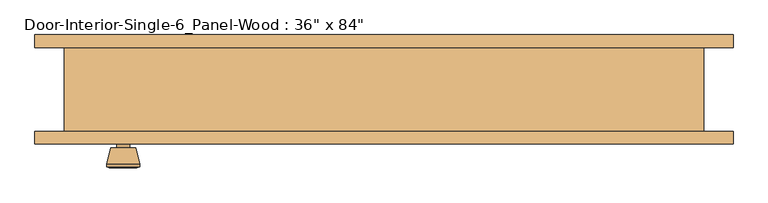
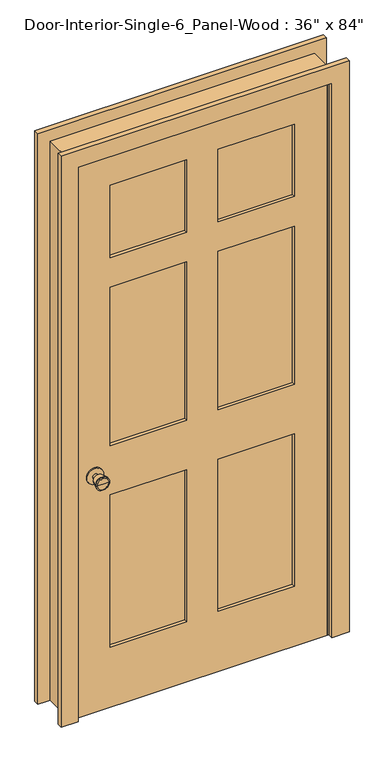
"""IFC4 building model written with IfcOpenShell, lengths in millimetres: door geometry."""

from ifc_helpers import new_model, si_unit, point, frame, frame_2d, origin, place, context, project, spatial, polyline, circle_curve, trimmed, segment, composite_curve, outline, extrude, faceted_brep, source, transform, mapped, element, save
from ifc_brep_helpers import plane_surface, cylinder_surface, revolved_surface, advanced_brep


def door_c610b25b(model_context):
    return source(origin(), model_context, "Body", "SolidModel", [
        advanced_brep(
        [(-393.7, -19.4, 914.4), (-403.7, -19.4, 914.4), (-383.7, -19.4, 914.4), (-373.2241324, 29.6, 914.4), (-414.1758676, 29.6, 914.4), (-393.7, 29.6, 914.4), (-368.7, 27.7721319, 914.4), (-418.7, 27.7721319, 914.4), (-368.7, 24.3084537, 914.4), (-418.7, 24.3084537, 914.4), (-375.063764, -0.4, 914.4), (-412.336236, -0.4, 914.4), (-383.7, -0.4, 914.4), (-403.7, -0.4, 914.4)],
        [
            (0, 1),
            (1, 2, circle_curve(frame((-393.7, -19.4, 914.4), z_axis=(0.0, -1.0, 0.0), x_axis=(-1.0, 0.0, 0.0)), 10.0)),
            (2, 0),
            (2, 1, circle_curve(frame((-393.7, -19.4, 914.4), z_axis=(0.0, -1.0, 0.0), x_axis=(-1.0, 0.0, 0.0)), 10.0)),
            (3, 4, circle_curve(frame((-393.7, 29.6, 914.4), z_axis=(0.0, 1.0, 0.0), x_axis=(-1.0, 0.0, 0.0)), 20.4758676)),
            (4, 5),
            (5, 3),
            (4, 3, circle_curve(frame((-393.7, 29.6, 914.4), z_axis=(0.0, 1.0, 0.0), x_axis=(-1.0, 0.0, 0.0)), 20.4758676)),
            (6, 7, circle_curve(frame((-393.7, 27.7721319, 914.4), z_axis=(0.0, 1.0, 0.0), x_axis=(-1.0, 0.0, 0.0)), 25.0)),
            (7, 4),
            (3, 6),
            (7, 6, circle_curve(frame((-393.7, 27.7721319, 914.4), z_axis=(0.0, 1.0, 0.0), x_axis=(-1.0, 0.0, 0.0)), 25.0)),
            (8, 9, circle_curve(frame((-393.7, 24.3084537, 914.4), z_axis=(0.0, 1.0, 0.0), x_axis=(-1.0, 0.0, 0.0)), 25.0)),
            (9, 7),
            (6, 8),
            (9, 8, circle_curve(frame((-393.7, 24.3084537, 914.4), z_axis=(0.0, 1.0, 0.0), x_axis=(-1.0, 0.0, 0.0)), 25.0)),
            (10, 11, circle_curve(frame((-393.7, -0.4, 914.4), z_axis=(0.0, 1.0, 0.0), x_axis=(-1.0, 0.0, 0.0)), 18.636236)),
            (11, 9),
            (8, 10),
            (11, 10, circle_curve(frame((-393.7, -0.4, 914.4), z_axis=(0.0, 1.0, 0.0), x_axis=(-1.0, 0.0, 0.0)), 18.636236)),
            (12, 13, circle_curve(frame((-393.7, -0.4, 914.4), z_axis=(0.0, 1.0, 0.0), x_axis=(-1.0, 0.0, 0.0)), 10.0)),
            (13, 11),
            (10, 12),
            (13, 12, circle_curve(frame((-393.7, -0.4, 914.4), z_axis=(0.0, 1.0, 0.0), x_axis=(-1.0, 0.0, 0.0)), 10.0)),
            (1, 13),
            (12, 2),
        ],
        [
            plane_surface(frame((-393.7, -19.4, 914.4), z_axis=(0.0, -1.0, 0.0), x_axis=(-1.0, 0.0, 0.0))),
            plane_surface(frame((-393.7, 29.6, 914.4), z_axis=(0.0, 1.0, 0.0), x_axis=(-1.0, 0.0, 0.0))),
            revolved_surface(polyline([(-414.1758676, 29.6, 914.4), (-418.7, 27.7721319, 914.4)]), (-393.7, -19.4, 914.4), (0.0, -1.0, 0.0)),
            cylinder_surface(frame((-393.7, -19.4, 914.4), z_axis=(0.0, -1.0, 0.0), x_axis=(-1.0, 0.0, 0.0)), 25.0),
            revolved_surface(polyline([(-418.7, 24.3084537, 914.4), (-412.336236, -0.4, 914.4)]), (-393.7, -19.4, 914.4), (0.0, -1.0, 0.0)),
            plane_surface(frame((-393.7, -0.4, 914.4), z_axis=(0.0, -1.0, 0.0), x_axis=(-1.0, 0.0, 0.0))),
            cylinder_surface(frame((-393.7, -19.4, 914.4), z_axis=(0.0, -1.0, 0.0), x_axis=(-1.0, 0.0, 0.0)), 10.0),
        ],
        [
            (0, [[1, 2, 3]]),
            (0, [[-3, 4, -1]]),
            (1, [[5, 6, 7]]),
            (1, [[8, -7, -6]]),
            (2, [[9, 10, -5, 11]]),
            (2, [[12, -11, -8, -10]]),
            (3, [[13, 14, -9, 15]]),
            (3, [[16, -15, -12, -14]]),
            (4, [[17, 18, -13, 19]]),
            (4, [[20, -19, -16, -18]]),
            (5, [[21, 22, -17, 23]]),
            (5, [[24, -23, -20, -22]]),
            (6, [[-2, 25, -21, 26]]),
            (6, [[-4, -26, -24, -25]]),
        ],
    ),
        extrude(outline(composite_curve([segment(trimmed(circle_curve(frame_2d((914.4, -393.7)), 30.0), [point((914.4, -423.7))], [point((914.4, -363.7))], False, "CARTESIAN"), True, "CONTINUOUS"), segment(trimmed(circle_curve(frame_2d((914.4, -393.7)), 30.0), [point((914.4, -363.7))], [point((914.4, -423.7))], False, "CARTESIAN"), True, "CONTINUOUS")], self_intersect=False)), frame((0.0, -25.4, 0.0), z_axis=(0.0, 1.0, 0.0), x_axis=(0.0, 0.0, 1.0)), (0.0, 0.0, 1.0), 6.0),
        advanced_brep(
        [(-393.7, -66.325, 914.4), (-383.7, -66.325, 914.4), (-403.7, -66.325, 914.4), (-373.2241324, -115.325, 914.4), (-393.7, -115.325, 914.4), (-414.1758676, -115.325, 914.4), (-368.7, -113.4971319, 914.4), (-418.7, -113.4971319, 914.4), (-368.7, -110.0334537, 914.4), (-418.7, -110.0334537, 914.4), (-375.063764, -85.325, 914.4), (-412.336236, -85.325, 914.4), (-383.7, -85.325, 914.4), (-403.7, -85.325, 914.4)],
        [
            (0, 1),
            (1, 2, circle_curve(frame((-393.7, -66.325, 914.4), z_axis=(0.0, 1.0, 0.0), x_axis=(-1.0, 0.0, 0.0)), 10.0)),
            (2, 0),
            (2, 1, circle_curve(frame((-393.7, -66.325, 914.4), z_axis=(0.0, 1.0, 0.0), x_axis=(-1.0, 0.0, 0.0)), 10.0)),
            (3, 4),
            (4, 5),
            (5, 3, circle_curve(frame((-393.7, -115.325, 914.4), z_axis=(0.0, -1.0, 0.0), x_axis=(-1.0, 0.0, 0.0)), 20.4758676)),
            (3, 5, circle_curve(frame((-393.7, -115.325, 914.4), z_axis=(0.0, -1.0, 0.0), x_axis=(-1.0, 0.0, 0.0)), 20.4758676)),
            (6, 3),
            (5, 7),
            (7, 6, circle_curve(frame((-393.7, -113.4971319, 914.4), z_axis=(0.0, -1.0, 0.0), x_axis=(-1.0, 0.0, 0.0)), 25.0)),
            (6, 7, circle_curve(frame((-393.7, -113.4971319, 914.4), z_axis=(0.0, -1.0, 0.0), x_axis=(-1.0, 0.0, 0.0)), 25.0)),
            (8, 6),
            (7, 9),
            (9, 8, circle_curve(frame((-393.7, -110.0334537, 914.4), z_axis=(0.0, -1.0, 0.0), x_axis=(-1.0, 0.0, 0.0)), 25.0)),
            (8, 9, circle_curve(frame((-393.7, -110.0334537, 914.4), z_axis=(0.0, -1.0, 0.0), x_axis=(-1.0, 0.0, 0.0)), 25.0)),
            (10, 8),
            (9, 11),
            (11, 10, circle_curve(frame((-393.7, -85.325, 914.4), z_axis=(0.0, -1.0, 0.0), x_axis=(-1.0, 0.0, 0.0)), 18.636236)),
            (10, 11, circle_curve(frame((-393.7, -85.325, 914.4), z_axis=(0.0, -1.0, 0.0), x_axis=(-1.0, 0.0, 0.0)), 18.636236)),
            (12, 10),
            (11, 13),
            (13, 12, circle_curve(frame((-393.7, -85.325, 914.4), z_axis=(0.0, -1.0, 0.0), x_axis=(-1.0, 0.0, 0.0)), 10.0)),
            (12, 13, circle_curve(frame((-393.7, -85.325, 914.4), z_axis=(0.0, -1.0, 0.0), x_axis=(-1.0, 0.0, 0.0)), 10.0)),
            (1, 12),
            (13, 2),
        ],
        [
            plane_surface(frame((-393.7, -66.325, 914.4), z_axis=(0.0, 1.0, 0.0), x_axis=(-1.0, 0.0, 0.0))),
            plane_surface(frame((-393.7, -115.325, 914.4), z_axis=(0.0, -1.0, 0.0), x_axis=(-1.0, 0.0, 0.0))),
            revolved_surface(polyline([(-414.1758676, -115.325, 914.4), (-418.7, -113.4971319, 914.4)]), (-393.7, -66.325, 914.4), (0.0, 1.0, 0.0)),
            cylinder_surface(frame((-393.7, -66.325, 914.4), z_axis=(0.0, 1.0, 0.0), x_axis=(-1.0, 0.0, 0.0)), 25.0),
            revolved_surface(polyline([(-418.7, -110.0334537, 914.4), (-412.336236, -85.325, 914.4)]), (-393.7, -66.325, 914.4), (0.0, 1.0, 0.0)),
            plane_surface(frame((-393.7, -85.325, 914.4), z_axis=(0.0, 1.0, 0.0), x_axis=(-1.0, 0.0, 0.0))),
            cylinder_surface(frame((-393.7, -66.325, 914.4), z_axis=(0.0, 1.0, 0.0), x_axis=(-1.0, 0.0, 0.0)), 10.0),
        ],
        [
            (0, [[1, 2, 3]]),
            (0, [[-3, 4, -1]]),
            (1, [[5, 6, 7]]),
            (1, [[-6, -5, 8]]),
            (2, [[9, -7, 10, 11]]),
            (2, [[-10, -8, -9, 12]]),
            (3, [[13, -11, 14, 15]]),
            (3, [[-14, -12, -13, 16]]),
            (4, [[17, -15, 18, 19]]),
            (4, [[-18, -16, -17, 20]]),
            (5, [[21, -19, 22, 23]]),
            (5, [[-22, -20, -21, 24]]),
            (6, [[25, -23, 26, -2]]),
            (6, [[-26, -24, -25, -4]]),
        ],
    ),
        extrude(outline(composite_curve([segment(trimmed(circle_curve(frame_2d((914.4, -393.7)), 30.0), [point((914.4, -423.7))], [point((914.4, -363.7))], False, "CARTESIAN"), True, "CONTINUOUS"), segment(trimmed(circle_curve(frame_2d((914.4, -393.7)), 30.0), [point((914.4, -363.7))], [point((914.4, -423.7))], False, "CARTESIAN"), True, "CONTINUOUS")], self_intersect=False)), frame((0.0, -66.325, 0.0), z_axis=(0.0, 1.0, 0.0), x_axis=(0.0, 0.0, 1.0)), (0.0, 0.0, 1.0), 6.0),
        faceted_brep([(482.6, -60.325, 0.0), (457.2, -60.325, 0.0), (457.2, -25.4, 0.0), (444.5, -25.4, 0.0), (444.5, 9.525, 0.0), (457.2, 9.525, 0.0), (457.2, 66.675, 0.0), (482.6, 66.675, 0.0), (482.6, 66.675, 2159.0), (482.6, -60.325, 2159.0), (457.2, 66.675, 2133.6), (-457.2, 66.675, 2133.6), (-457.2, 66.675, 0.0), (-482.6, 66.675, 0.0), (-482.6, 66.675, 2159.0), (457.2, 9.525, 2133.6), (444.5, 9.525, 2120.9), (-444.5, 9.525, 2120.9), (-444.5, 9.525, 0.0), (-457.2, 9.525, 0.0), (-457.2, 9.525, 2133.6), (444.5, -25.4, 2120.9), (457.2, -25.4, 2133.6), (-457.2, -25.4, 2133.6), (-457.2, -25.4, 0.0), (-444.5, -25.4, 0.0), (-444.5, -25.4, 2120.9), (457.2, -60.325, 2133.6), (-482.6, -60.325, 2159.0), (-482.6, -60.325, 0.0), (-457.2, -60.325, 0.0), (-457.2, -60.325, 2133.6)], [[[0, 1, 2, 3, 4, 5, 6, 7]], [[7, 8, 9, 0]], [[6, 10, 11, 12, 13, 14, 8, 7]], [[5, 15, 10, 6]], [[4, 16, 17, 18, 19, 20, 15, 5]], [[3, 21, 16, 4]], [[2, 22, 23, 24, 25, 26, 21, 3]], [[1, 27, 22, 2]], [[0, 9, 28, 29, 30, 31, 27, 1]], [[8, 14, 28, 9]], [[15, 20, 11, 10]], [[21, 26, 17, 16]], [[27, 31, 23, 22]], [[29, 13, 12, 19, 18, 25, 24, 30]], [[14, 13, 29, 28]], [[20, 19, 12, 11]], [[26, 25, 18, 17]], [[31, 30, 24, 23]]]),
        extrude(outline(polyline([(2133.6, -457.2), (0.0, -457.2), (0.0, 457.2), (2133.6, 457.2), (2133.6, -457.2)]), holes=[polyline([(2014.5375, 57.15), (2014.5375, 336.55), (1735.1375, 336.55), (1735.1375, 57.15), (2014.5375, 57.15)]), polyline([(1620.8375, 336.55), (1009.65, 336.55), (1009.65, 57.15), (1620.8375, 57.15), (1620.8375, 336.55)]), polyline([(1009.65, -57.15), (1009.65, -336.55), (1620.8375, -336.55), (1620.8375, -57.15), (1009.65, -57.15)]), polyline([(1735.1375, -336.55), (2014.5375, -336.55), (2014.5375, -57.15), (1735.1375, -57.15), (1735.1375, -336.55)]), polyline([(819.15, 57.15), (819.15, 336.55), (231.775, 336.55), (231.775, 57.15), (819.15, 57.15)]), polyline([(231.775, -57.15), (231.775, -336.55), (819.15, -336.55), (819.15, -57.15), (231.775, -57.15)])]), frame((0.0, -60.325, 0.0), z_axis=(0.0, 1.0, 0.0), x_axis=(0.0, 0.0, 1.0)), (0.0, 0.0, 1.0), 34.925),
        extrude(outline(polyline([(336.55, -37.0416667), (336.55, -48.6833333), (57.15, -48.6833333), (57.15, -37.0416667), (336.55, -37.0416667)])), frame((0.0, 0.0, 1735.1375), z_axis=(0.0, 0.0, 1.0), x_axis=(1.0, 0.0, 0.0)), (0.0, 0.0, 1.0), 279.4),
        extrude(outline(polyline([(336.55, -37.0416667), (336.55, -48.6833333), (57.15, -48.6833333), (57.15, -37.0416667), (336.55, -37.0416667)])), frame((0.0, 0.0, 1009.65), z_axis=(0.0, 0.0, 1.0), x_axis=(1.0, 0.0, 0.0)), (0.0, 0.0, 1.0), 611.1875),
        extrude(outline(polyline([(-57.15, -37.0416667), (-57.15, -48.6833333), (-336.55, -48.6833333), (-336.55, -37.0416667), (-57.15, -37.0416667)])), frame((0.0, 0.0, 1009.65), z_axis=(0.0, 0.0, 1.0), x_axis=(1.0, 0.0, 0.0)), (0.0, 0.0, 1.0), 611.1875),
        extrude(outline(polyline([(-57.15, -37.0416667), (-57.15, -48.6833333), (-336.55, -48.6833333), (-336.55, -37.0416667), (-57.15, -37.0416667)])), frame((0.0, 0.0, 1735.1375), z_axis=(0.0, 0.0, 1.0), x_axis=(1.0, 0.0, 0.0)), (0.0, 0.0, 1.0), 279.4),
        extrude(outline(polyline([(336.55, -37.0416667), (336.55, -48.6833333), (57.15, -48.6833333), (57.15, -37.0416667), (336.55, -37.0416667)])), frame((0.0, 0.0, 231.775), z_axis=(0.0, 0.0, 1.0), x_axis=(1.0, 0.0, 0.0)), (0.0, 0.0, 1.0), 587.375),
        extrude(outline(polyline([(-57.15, -37.0416667), (-57.15, -48.6833333), (-336.55, -48.6833333), (-336.55, -37.0416667), (-57.15, -37.0416667)])), frame((0.0, 0.0, 231.775), z_axis=(0.0, 0.0, 1.0), x_axis=(1.0, 0.0, 0.0)), (0.0, 0.0, 1.0), 587.375),
        extrude(outline(polyline([(0.0, 527.05), (2203.45, 527.05), (2203.45, -527.05), (0.0, -527.05), (0.0, -463.55), (2139.95, -463.55), (2139.95, 463.55), (0.0, 463.55), (0.0, 527.05)])), frame((0.0, -79.375, 0.0), z_axis=(0.0, 1.0, 0.0), x_axis=(0.0, 0.0, 1.0)), (0.0, 0.0, 1.0), 19.05),
        extrude(outline(polyline([(0.0, 527.05), (2203.45, 527.05), (2203.45, -527.05), (0.0, -527.05), (0.0, -463.55), (2139.95, -463.55), (2139.95, 463.55), (0.0, 463.55), (0.0, 527.05)])), frame((0.0, 66.675, 0.0), z_axis=(0.0, 1.0, 0.0), x_axis=(0.0, 0.0, 1.0)), (0.0, 0.0, 1.0), 19.05),
    ])


if __name__ == "__main__":
    model = new_model("IFC4")
    model_context = context("Model", 3, world=origin())
    ifc_project = project(units=[si_unit("LENGTHUNIT", "METRE", prefix="MILLI")], contexts=[model_context])
    site = spatial("IfcSite", under=ifc_project)
    building = spatial("IfcBuilding", under=site)
    placement = place(None, origin())
    door_shape = door_c610b25b(model_context)
    element("IfcDoor", 1, ObjectType="Door-Interior-Single-6_Panel-Wood : 36\" x 84\"", at=placement, inside=building, context=model_context, shape_type="MappedRepresentation", body=[
        mapped(door_shape, transform((0.0, 0.0, 0.0), x_axis=(1.0, 0.0, 0.0), y_axis=(0.0, 1.0, 0.0), z_axis=(0.0, 0.0, 1.0))),
    ])
    save(model, "model.ifc")

# Revit data of these elements
# Type "Door-Interior-Single-6_Panel-Wood : 36\" x 84\""
#   Type Mark = "8"
#   Assembly Code = "C1020300"
#   Analytic Construction = "Wooden"
#   Top Rail = 0' - 4 11/16"
#   Top Panel = 0' - 11"
#   Thickness = 0' - 1 3/8"
#   Thermal Resistance (R) = 2.5876 (h·ft²·°F)/BTU
#   Swing Angle [instance default] = 90.00°
#   Stiles = 0' - 4 3/4"
#   Rough Width = 3' - 2"
#   Rough Height = 7' - 1"
#   Mullion = 0' - 4 1/2"
#   Lock Rail = 0' - 7 1/2"
#   Intermediate Rail = 0' - 4 1/2"
#   Height = 7' - 0"
#   Width = 3' - 0"
#   Heat Transfer Coefficient (U) = 0.3865 BTU/(h·ft²·°F)
#   Bottom Rail = 0' - 9 1/8"
#   Trim Material = Cherry
#   Panel Material = Cherry
#   Frame Material = Cherry
#   Door Handle Material = Aluminum
#   Visual Light Transmittance = 0
#   Solar Heat Gain Coefficient = 0
#   Wall Closure = (empty or 0)
#   Function = (empty or 0)
# Element 1 (IfcDoor, "Door-Interior-Single-6_Panel-Wood : 36\" x 84\"")
#   Materials on its faces: "Cherry", "Aluminum"
# Materials
#   "Cherry": class "Wood", colour RGB 226 177 128, transparency 0, Description = "Prunus Serotina", Cost = 0
#   "Aluminum": class "Metal", colour RGB 247 247 247, transparency 0, Description = "Aluminum 6061", Cost = 0
